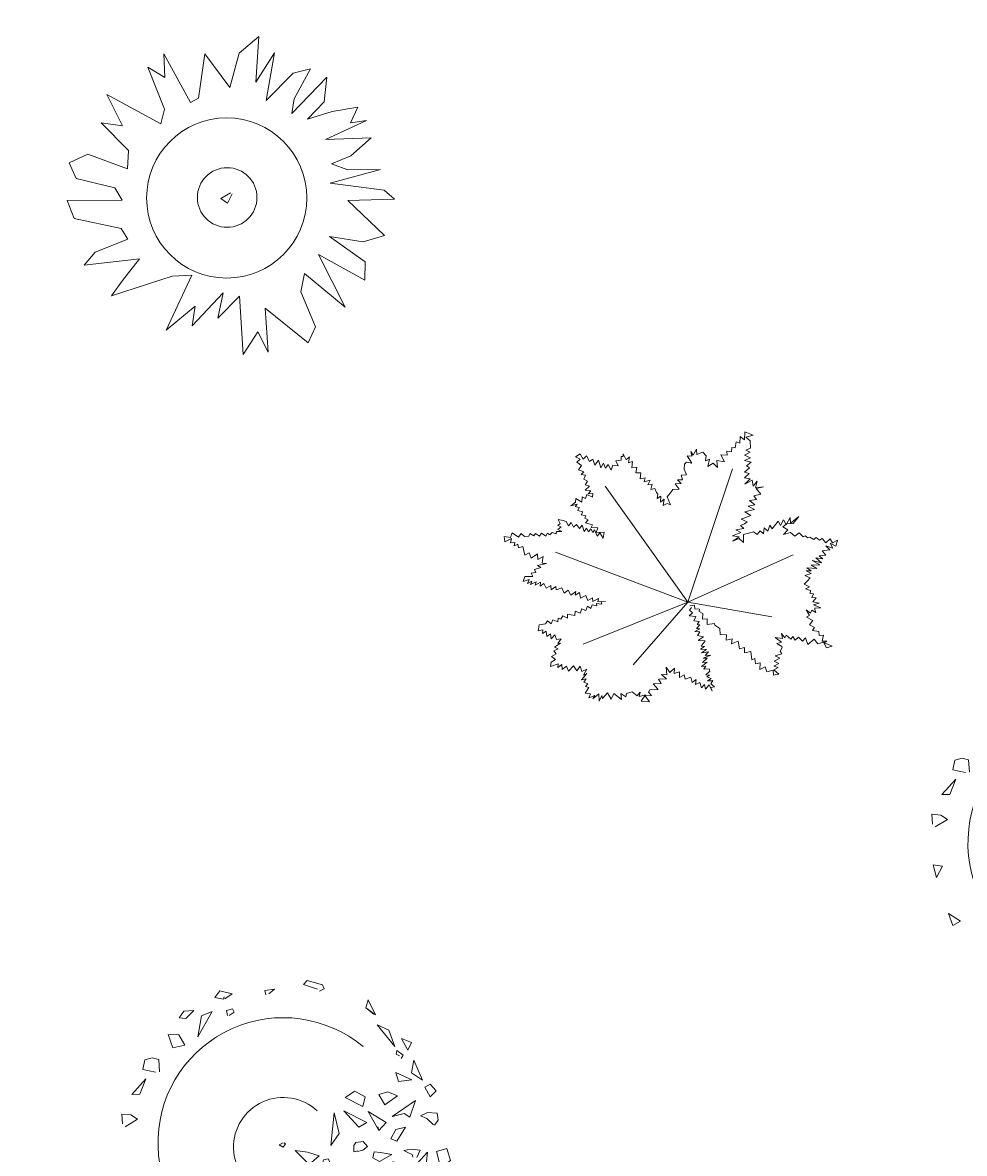
# Model space of a CAD drawing. Units: inches. Extents: x 8049 to 8459, y 820 to 1350.
# Tile 6 of 25: x 8109 to 8132, y 877 to 905. Entities that reach past the tile are written whole.
import ezdxf

# ---------------------------------------------------------------- set-up
doc = ezdxf.new("R2010")
doc.units = ezdxf.units.IN
doc.header["$MEASUREMENT"] = 0
doc.layers.add('A-ANNO-DIMS', color=2, linetype='Continuous', lineweight=18)
doc.layers.add('zelen', color=69, linetype='Continuous', lineweight=13)
doc.styles.get("Standard").update_dxf_attribs({"font": 'arial.ttf'})
doc.dimstyles.get("Standard").update_dxf_attribs({"dimtxt": 0.18, "dimasz": 0.18, "dimexe": 0.18, "dimexo": 0.0625, "dimgap": 0.09, "dimtad": 0, "dimtih": 1, "dimtoh": 1, "dimdec": 4, "dimzin": 0, "dimdsep": 46, "dimtxsty": 'Standard', "dimcen": 0.09, "dimadec": 0, "dimazin": 0, "dimtfac": 1, "dimtdec": 4, "dimtofl": 0, "dimtmove": 0, "dimatfit": 3, "dimfxl": 1, "dimtolj": 1, "dimtzin": 0, "dimarcsym": 0})

# ---------------------------------------------------------------- blocks, each defined once
blk = doc.blocks.new('z_74')
for p, q in [((34.4, 446.7), (93.3, 497)), ((93.3, 497), (83.9, 360.3)), ((-189.4, 445.2), (-110.2, 299.7)), ((-186.5, 374.9), (-189.4, 445.2)), ((-86.8, 312.7), (-67.9, 445.2)), ((-67.9, 445.2), (6.7, 344.6)), ((6.7, 344.6), (34.4, 446.7)), ((83.9, 360.3), (139.6, 447.9)), ((139.6, 447.9), (115.1, 306.1)), ((-237.2, 405.2), (-186.5, 374.9)), ((-188, 280), (-237.2, 405.2)), ((115.1, 306.1), (195.3, 387)), ((191.5, 267.3), (295.2, 375.5)), ((195.3, 387), (247.1, 400.9)), ((247.1, 400.9), (198.5, 310.6)), ((295.2, 375.5), (287.6, 302.1)), ((-359.3, 324.3), (-198.2, 236.1)), ((-312.4, 230.9), (-359.3, 324.3)), ((-110.2, 299.7), (-86.8, 312.7)), ((198.5, 310.6), (191.5, 267.3)), ((-198.2, 236.1), (-188, 280)), ((287.6, 302.1), (238.4, 250.6)), ((238.4, 250.6), (311, 273.7)), ((311, 273.7), (388.2, 286.7)), ((388.2, 286.7), (366, 239.7)), ((-375.9, 239.1), (-312.4, 230.9)), ((-294.6, 157.3), (-375.9, 239.1)), ((413.3, 247), (291.4, 189.7)), ((366, 239.7), (413.3, 247)), ((291.4, 189.7), (427.5, 195.2)), ((427.5, 195.2), (367.5, 141.5)), ((-471.8, 120.9), (-415.6, 146.1)), ((-415.6, 146.1), (-297.6, 102.4)), ((-297.6, 102.4), (-294.6, 157.3)), ((367.5, 141.5), (309.2, 117.3)), ((-450.8, 73.9), (-471.8, 120.9)), ((309.2, 117.3), (358.2, 99.1)), ((-335.1, 45.8), (-450.8, 73.9)), ((455.8, 100.6), (305.4, 59.4)), ((358.2, 99.1), (455.8, 100.6)), ((-313.9, 9.1), (-335.1, 45.8)), ((305.4, 59.4), (466, 38.8)), ((466, 38.8), (497.2, 12.1)), ((-477.4, 8.2), (-313.9, 9.1)), ((-456.4, -45.8), (-477.4, 8.2)), ((8.7, 30.9), (-19.5, 13.9)), ((-19.5, 13.9), (0, 0)), ((0, 0), (13.4, 27.9)), ((497.2, 12.1), (358.2, 8.5)), ((358.2, 8.5), (467.2, -96.1)), ((-316.8, -75.2), (-456.4, -45.8)), ((-296.4, -106.7), (-316.8, -75.2)), ((303.7, -98.8), (410, -174.6)), ((403.6, -114.9), (303.7, -98.8)), ((467.2, -96.1), (403.6, -114.9)), ((-393.7, -146.1), (-296.4, -106.7)), ((-426.7, -184.3), (-393.7, -146.1)), ((-262.6, -165.2), (-426.7, -184.3)), ((-312.7, -229.7), (-262.6, -165.2)), ((271.3, -152.4), (350, -309.1)), ((408.9, -228.8), (271.3, -152.4)), ((410, -174.6), (408.9, -228.8)), ((-165.2, -217.6), (-345.3, -276.1)), ((-345.3, -276.1), (-312.7, -229.7)), ((-182.4, -377.6), (-106.4, -213.9)), ((-106.4, -213.9), (-165.2, -217.6)), ((229.6, -209.7), (218, -264.3)), ((350, -309.1), (229.6, -209.7)), ((-13.1, -266.4), (-105.5, -365.5)), ((-28.9, -341.8), (-13.1, -266.4)), ((218, -264.3), (262, -367.6)), ((35.8, -276.7), (-28.9, -341.8)), ((46.6, -450.6), (35.8, -276.7)), ((-96.5, -306.1), (-182.4, -377.6)), ((-105.5, -365.5), (-96.5, -306.1)), ((111.6, -312.4), (120.9, -443.4)), ((240.1, -415.5), (111.6, -312.4)), ((262, -367.6), (240.1, -415.5)), ((90.1, -383.4), (46.6, -450.6)), ((120.9, -443.4), (90.1, -383.4))]:
    blk.add_line(p, q)
for centre, radius in [((-2.5, 15.8), 238.5), ((-1.1, 17.1), 88.8)]:
    blk.add_circle(centre, radius)
blk = doc.blocks.new('z_85')
for p, q in [((168.5, 483.9), (169.7, 507.5)), ((169.7, 507.5), (194.7, 497.5)), ((140.4, 459.9), (144.1, 478.3)), ((144.1, 478.3), (154.8, 474.2)), ((154.8, 474.2), (155.6, 493.8)), ((155.6, 493.8), (168.5, 483.9)), ((194.7, 497.5), (173, 491.4)), ((173, 491.4), (185.2, 481.2)), ((185.2, 481.2), (186.9, 458.5)), ((-334.5, 433), (-320.5, 441.8)), ((-320.5, 441.8), (-312.2, 426.3)), ((-192.6, 433.8), (-192.5, 442.2)), ((-192.5, 442.2), (-183.3, 424.5)), ((8.4, 449), (15.4, 438)), ((11.7, 434.9), (8.4, 449)), ((15.4, 438), (25.6, 455.6)), ((25.6, 455.6), (26.4, 439.7)), ((26.4, 439.7), (44.1, 447.4)), ((44.1, 447.4), (54.4, 436.3)), ((98.5, 438.8), (116.6, 438)), ((108.9, 418.4), (98.5, 438.8)), ((116.1, 450.2), (130, 447.6)), ((116.6, 438), (116.1, 450.2)), ((130, 447.6), (130.9, 460.7)), ((130.9, 460.7), (140.4, 459.9)), ((185.1, 447.3), (169, 438)), ((169, 438), (186.4, 430.3)), ((186.9, 458.5), (172.1, 453.2)), ((172.1, 453.2), (185.1, 447.3)), ((-320.3, 426.3), (-334.5, 433)), ((-331, 417), (-320.3, 426.3)), ((-316.9, 407.2), (-331, 417)), ((-325.3, 394.5), (-316.9, 407.2)), ((-312.2, 426.3), (-302, 436.4)), ((-302, 436.4), (-292.5, 418.9)), ((-292.5, 418.9), (-282.7, 426.1)), ((-282.7, 426.1), (-277, 408.1)), ((-277, 408.1), (-266.3, 423.5)), ((-266.3, 423.5), (-258.7, 400.7)), ((-258.7, 400.7), (-250.8, 414.2)), ((-250.8, 414.2), (-244.9, 399.8)), ((-244.9, 399.8), (-237.2, 410.8)), ((-237.2, 410.8), (-228.5, 393.9)), ((-228.5, 393.9), (-223.5, 408.6)), ((-223.5, 408.6), (-207.8, 406.4)), ((-214.2, 421.3), (-198.5, 423)), ((-207.8, 406.4), (-214.2, 421.3)), ((-198.5, 423), (-198.2, 434.1)), ((-198.2, 434.1), (-192.6, 433.8)), ((-183.3, 424.5), (-173.3, 433.2)), ((-173.3, 433.2), (-176.4, 415.5)), ((-176.4, 415.5), (-165.1, 418.9)), ((-165.1, 418.9), (-166.4, 400.3)), ((-10.8, 396), (-9.6, 410.9)), ((-9.6, 410.9), (-3.8, 416.9)), ((-3.8, 416.9), (11.4, 414.5)), ((-2.1, 435.8), (11.7, 434.9)), ((11.4, 414.5), (-2.1, 435.8)), ((54.4, 436.3), (52.3, 421.7)), ((52.3, 421.7), (64.6, 426)), ((64.6, 426), (59.8, 403.9)), ((59.8, 403.9), (75.6, 414.2)), ((75.6, 414.2), (88.3, 401.4)), ((86.4, 422.5), (108.9, 418.4)), ((88.3, 401.4), (86.4, 422.5)), ((186.4, 430.3), (169.1, 422.7)), ((169.1, 422.7), (188.1, 417.5)), ((188.1, 417.5), (174.5, 406.5)), ((174.5, 406.5), (183.6, 400.7)), ((-309.5, 388.7), (-325.3, 394.5)), ((-317.2, 380.4), (-309.5, 388.7)), ((-305.1, 378.2), (-317.2, 380.4)), ((-309.5, 366.8), (-305.1, 378.2)), ((-166.4, 400.3), (-152.4, 402.8)), ((-152.4, 402.8), (-154.8, 385.2)), ((-154.8, 385.2), (-139.8, 385.6)), ((-139.8, 385.6), (-142, 367.5)), ((-142, 367.5), (-126.8, 370.7)), ((-126.8, 370.7), (-129.7, 358.9)), ((-19.9, 378.2), (-4.1, 379.1)), ((-16.4, 364.7), (-19.9, 378.2)), ((-4.1, 379.1), (-10.8, 396)), ((0, 0), (132.7, 397)), ((182.7, 383.5), (168.5, 371)), ((168.5, 371), (185.5, 367.5)), ((183.6, 400.7), (169.1, 387.1)), ((169.1, 387.1), (182.7, 383.5)), ((-299.2, 360.3), (-309.5, 366.8)), ((-305.9, 349.8), (-299.2, 360.3)), ((-292.6, 345.9), (-305.9, 349.8)), ((-305.3, 333.9), (-292.6, 345.9)), ((0, 0), (-245.8, 345.3)), ((-129.7, 358.9), (-112.6, 364.1)), ((-112.6, 364.1), (-118.7, 349.7)), ((-118.7, 349.7), (-106.5, 351.7)), ((-106.5, 351.7), (-110.4, 335.8)), ((-110.4, 335.8), (-98.6, 339.2)), ((-98.6, 339.2), (-92.9, 326.8)), ((-45, 336.2), (-26.1, 337)), ((-37.5, 352.7), (-19.6, 354.2)), ((-26.1, 337), (-37.5, 352.7)), ((-31.2, 364.3), (-16.4, 364.7)), ((-19.6, 354.2), (-31.2, 364.3)), ((185.5, 367.5), (169.7, 351.3)), ((169.7, 351.3), (191.1, 364.1)), ((191.1, 364.1), (194, 345.3)), ((194, 345.3), (206.3, 360.8)), ((206.3, 360.8), (201.7, 341.2)), ((201.7, 341.2), (224.8, 344.2)), ((224.8, 344.2), (203.2, 339.2)), ((203.2, 339.2), (217.5, 321.8)), ((-334.3, 298.5), (-333.4, 308.7)), ((-333.4, 308.7), (-315.2, 298.3)), ((-315.2, 298.3), (-314.9, 314.1)), ((-314.9, 314.1), (-305, 309.4)), ((-288.9, 332.3), (-305.3, 333.9)), ((-305, 309.4), (-300.9, 321)), ((-300.9, 321), (-284.3, 312.7)), ((-296.8, 323.1), (-288.9, 332.3)), ((-283.1, 324), (-296.8, 323.1)), ((-284.3, 312.7), (-283.1, 324)), ((-92.9, 326.8), (-89.6, 322.3)), ((-89.6, 322.3), (-91.1, 309)), ((-91.1, 309), (-80.4, 316.3)), ((-80.4, 316.3), (-81.2, 298.5)), ((-81.2, 298.5), (-70.2, 306.6)), ((-70.2, 306.6), (-73.6, 287.8)), ((-61.6, 314), (-48.8, 329.6)), ((-51.7, 290.2), (-61.6, 314)), ((-48.8, 329.6), (-45, 336.2)), ((204.7, 306.3), (183.1, 303.2)), ((183.1, 303.2), (199.8, 290.5)), ((217.5, 321.8), (196.8, 317.3)), ((196.8, 317.3), (204.7, 306.3)), ((-348.8, 287.5), (-334.3, 298.5)), ((-329.7, 291.9), (-348.8, 287.5)), ((-335.7, 285.2), (-329.7, 291.9)), ((-323.9, 282.5), (-335.7, 285.2)), ((-327.7, 273.4), (-323.9, 282.5)), ((-312.5, 269.8), (-327.7, 273.4)), ((-318.1, 260.9), (-312.5, 269.8)), ((-73.6, 287.8), (-62, 294.6)), ((-62, 294.6), (-51.7, 290.2)), ((198, 276.2), (169.3, 269.4)), ((199.8, 290.5), (179.5, 286.4)), ((179.5, 286.4), (198, 276.2)), ((-386.6, 246.8), (-370.9, 243.8)), ((-380.3, 234.1), (-386.6, 246.8)), ((-370.9, 243.8), (-362.5, 240.1)), ((-362.5, 240.1), (-355.4, 227.7)), ((-355.4, 227.7), (-347.7, 237.1)), ((-347.7, 237.1), (-340.1, 223.9)), ((-303.5, 257.1), (-318.1, 260.9)), ((-306.9, 250.2), (-303.5, 257.1)), ((-296.5, 245.4), (-306.9, 250.2)), ((-304.8, 236.9), (-296.5, 245.4)), ((-284, 230.8), (-304.8, 236.9)), ((187.9, 258.2), (158.6, 247.3)), ((158.6, 247.3), (176.5, 239.3)), ((176.5, 239.3), (169.1, 234)), ((169.3, 269.4), (187.9, 258.2)), ((251.2, 218.3), (269.1, 241.8)), ((269.1, 241.8), (276.1, 228.2)), ((276.1, 228.2), (284.6, 245.4)), ((284.6, 245.4), (292.5, 230.8)), ((292.5, 230.8), (304.2, 252.6)), ((304.2, 252.6), (305.4, 235.8)), ((305.4, 235.8), (330.6, 255.3)), ((330.6, 255.3), (314, 234.4)), ((-527.9, 192.6), (-523, 206.4)), ((-523, 206.4), (-504.7, 194.2)), ((-504.7, 194.2), (-496.5, 204.8)), ((-496.5, 204.8), (-486, 196.2)), ((-473.8, 197.3), (-470.6, 205)), ((-470.6, 205), (-459, 197.9)), ((-459, 197.9), (-453.2, 204.7)), ((-453.2, 204.7), (-441.7, 197.3)), ((-441.7, 197.3), (-436, 206.1)), ((-436, 206.1), (-423, 196.7)), ((-423, 196.7), (-417.9, 205.5)), ((-417.9, 205.5), (-411.3, 200.8)), ((-411.3, 200.8), (-403.9, 207.3)), ((-403.9, 207.3), (-392, 203.9)), ((-392, 203.9), (-391, 210.5)), ((-391, 210.5), (-375.1, 210.9)), ((-387.5, 216.4), (-377.3, 224.9)), ((-375.1, 210.9), (-387.5, 216.4)), ((-387.2, 228.2), (-380.3, 234.1)), ((-377.3, 224.9), (-387.2, 228.2)), ((-340.1, 223.9), (-331.2, 232.1)), ((-331.2, 232.1), (-323, 219.9)), ((-323, 219.9), (-314.9, 229.4)), ((-314.9, 229.4), (-308.7, 210.5)), ((-308.7, 210.5), (-301.4, 220.5)), ((-301.4, 220.5), (-296.2, 209.5)), ((-296.2, 209.5), (-288.7, 218.5)), ((-288.7, 218.5), (-282.8, 208)), ((-287.5, 222.7), (-284, 230.8)), ((-267.9, 221.3), (-287.5, 222.7)), ((-282.8, 208), (-278.3, 215.3)), ((-278.3, 215.3), (-269.6, 197)), ((-272.7, 208.1), (-267.9, 221.3)), ((-249.1, 208.6), (-272.7, 208.1)), ((-269.6, 197), (-261.6, 206.7)), ((-261.6, 206.7), (-252.6, 191.1)), ((-252.6, 191.1), (-249.1, 208.6)), ((157.5, 207.7), (133, 198.3)), ((166.6, 220), (142.5, 215.8)), ((142.5, 215.8), (157.5, 207.7)), ((169.1, 234), (156.5, 228.6)), ((156.5, 228.6), (166.6, 220)), ((165.5, 178.4), (166.1, 202.2)), ((166.1, 202.2), (195.8, 210)), ((195.8, 210), (206.3, 202.3)), ((206.3, 202.3), (214.9, 212.7)), ((214.9, 212.7), (225, 203.7)), ((225, 203.7), (227.4, 221.4)), ((227.4, 221.4), (237.6, 211.9)), ((237.6, 211.9), (244, 229.6)), ((244, 229.6), (251.2, 218.3)), ((291.9, 231.3), (282.8, 224.3)), ((282.8, 224.3), (297.7, 215.3)), ((297.7, 215.3), (285.2, 201.4)), ((285.2, 201.4), (305.7, 207.8)), ((294, 233.8), (291.9, 231.3)), ((314, 234.4), (294, 233.8)), ((305.7, 207.8), (318.4, 196.7)), ((318.4, 196.7), (331.5, 207.2)), ((331.5, 207.2), (343.4, 195.3)), ((-547.4, 195.4), (-527.9, 192.6)), ((-544.7, 179.5), (-547.4, 195.4)), ((-524.7, 189.5), (-544.7, 179.5)), ((-528.5, 176.6), (-524.7, 189.5)), ((-515.5, 177.6), (-528.5, 176.6)), ((-516.7, 167.9), (-515.5, 177.6)), ((-506.3, 173.2), (-516.7, 167.9)), ((-504.7, 162.4), (-506.3, 173.2)), ((-486, 196.2), (-473.8, 197.3)), ((133, 198.3), (152.7, 194.8)), ((152.7, 194.8), (134.2, 181.8)), ((134.2, 181.8), (152.3, 190.3)), ((152.3, 190.3), (165.5, 178.4)), ((343.4, 195.3), (349.2, 197.8)), ((349.2, 197.8), (357.1, 191.7)), ((357.1, 191.7), (363.4, 194)), ((363.4, 194), (375.4, 187.3)), ((375.4, 187.3), (381.6, 192.9)), ((381.6, 192.9), (391.6, 185.1)), ((391.6, 185.1), (399.5, 189.8)), ((399.5, 189.8), (410.7, 177.1)), ((410.7, 177.1), (423.8, 189)), ((423.8, 189), (430.9, 177.3)), ((423.8, 175.6), (431.6, 161.5)), ((440.2, 166.6), (423.8, 175.6)), ((430.9, 177.3), (445.2, 185.4)), ((445.2, 185.4), (440.2, 166.6)), ((-491.4, 165.7), (-504.7, 162.4)), ((-484.9, 140.6), (-491.4, 165.7)), ((-472, 147), (-484.9, 140.6)), ((-466.4, 131.1), (-472, 147)), ((-447.4, 143.9), (-466.4, 131.1)), ((-446.4, 127.5), (-447.4, 143.9)), ((-431.2, 136.1), (-446.4, 127.5)), ((-432.5, 124.7), (-431.2, 136.1)), ((0, 0), (-394.4, 149.4)), ((0, 0), (313.9, 140.8)), ((410.7, 140.5), (391.1, 138)), ((391.1, 138), (402.3, 129)), ((422.9, 156), (399.8, 152.7)), ((399.8, 152.7), (410.7, 140.5)), ((410.7, 167.7), (422.9, 156)), ((431.6, 161.5), (410.7, 167.7)), ((-456.8, 97.3), (-437.9, 103.7)), ((-447.3, 109), (-420.9, 115.7)), ((-437.9, 103.7), (-447.3, 109)), ((-433.6, 116.8), (-432.5, 124.7)), ((-420.9, 115.7), (-433.6, 116.8)), ((354.4, 102.3), (367.3, 93.6)), ((384, 100.5), (354.4, 102.3)), ((392.9, 111.3), (367, 110.4)), ((367, 110.4), (384, 100.5)), ((370, 124.5), (392.9, 111.3)), ((397.4, 117.9), (370, 124.5)), ((380.7, 131.9), (397.4, 117.9)), ((402.3, 129), (380.7, 131.9)), ((-490.1, 61.5), (-485.7, 76.6)), ((-472.7, 67.7), (-490.1, 61.5)), ((-485.7, 76.6), (-461.1, 77.2)), ((-477.3, 56.2), (-472.7, 67.7)), ((-466.3, 86.6), (-452.6, 88.2)), ((-461.1, 77.2), (-466.3, 86.6)), ((-452.6, 88.2), (-456.8, 97.3)), ((367.5, 85.5), (348.2, 79.7)), ((348.2, 79.7), (364, 72.5)), ((367.3, 93.6), (352.7, 93.5)), ((352.7, 93.5), (367.5, 85.5)), ((364, 72.5), (355.3, 62.8)), ((-464.1, 63.3), (-477.3, 56.2)), ((-468.4, 52.6), (-464.1, 63.3)), ((-452, 61.1), (-468.4, 52.6)), ((-455.1, 51.2), (-452, 61.1)), ((-439, 59.8), (-455.1, 51.2)), ((-439.5, 47.5), (-439, 59.8)), ((-428.5, 56.1), (-439.5, 47.5)), ((-421.5, 42.4), (-428.5, 56.1)), ((-408.4, 49.5), (-421.5, 42.4)), ((-406.6, 37.3), (-408.4, 49.5)), ((-393.5, 46.8), (-406.6, 37.3)), ((-392.2, 37), (-393.5, 46.8)), ((-375.3, 43.4), (-392.2, 37)), ((-368.7, 27.4), (-375.3, 43.4)), ((-356.3, 36.3), (-368.7, 27.4)), ((-348.5, 20.8), (-356.3, 36.3)), ((355.3, 62.8), (346.4, 53.6)), ((346.4, 53.6), (362.3, 46.4)), ((362.3, 46.4), (350.4, 40.1)), ((350.4, 40.1), (365.4, 35.2)), ((365.4, 35.2), (364.6, 26)), ((-333.9, 32.3), (-348.5, 20.8)), ((-335.5, 21.5), (-333.9, 32.3)), ((-322.4, 29.1), (-335.5, 21.5)), ((-319.9, 12.2), (-322.4, 29.1)), ((-303.8, 20), (-319.9, 12.2)), ((0, 0), (-312.2, -125)), ((-297.7, 5.3), (-303.8, 20)), ((-284.2, 12.8), (-297.7, 5.3)), ((-282.8, 2.5), (-284.2, 12.8)), ((-266.1, 11.6), (-282.8, 2.5)), ((-268.5, 0.9), (-266.1, 11.6)), ((-245.2, 1.9), (-268.5, 0.9)), ((-258.6, 1.3), (-245.2, 1.9)), ((-256.6, -5.5), (-258.6, 1.3)), ((0, 0), (-163.1, -186)), ((0, 0), (249.7, -43.2)), ((364.6, 26), (373.9, 25.2)), ((373.9, 25.2), (368.8, 14.6)), ((368.8, 14.6), (381.5, 13.5)), ((381.5, 13.5), (372.3, 1.1)), ((372.3, 1.1), (390.8, -3.1)), ((-337, -39.8), (-335.4, -26.5)), ((-335.4, -26.5), (-320, -32.7)), ((-320, -32.7), (-316.6, -19.6)), ((-316.6, -19.6), (-303.5, -24.4)), ((-303.5, -24.4), (-299.1, -12.1)), ((-299.1, -12.1), (-288.4, -18.9)), ((-288.4, -18.9), (-284.9, -7.8)), ((-284.9, -7.8), (-270.6, -10.5)), ((-272, -3.8), (-256.6, -5.5)), ((-270.6, -10.5), (-272, -3.8)), ((14.2, -31.5), (3.8, -40.4)), ((11, -15.5), (4.4, -23.3)), ((4.4, -23.3), (14.2, -31.5)), ((19.4, -9.1), (6, -11.1)), ((20.6, -19.7), (19.4, -9.1)), ((34.5, -21), (20.6, -19.7)), ((33.9, -27.7), (34.5, -21)), ((44.7, -33.5), (33.9, -27.7)), ((43.2, -50.4), (44.7, -33.5)), ((352.1, -22.6), (362.5, -39.2)), ((365.2, -32.7), (352.1, -22.6)), ((368.7, -23.2), (365.2, -32.7)), ((380.7, -30.1), (368.7, -23.2)), ((390.8, -3.1), (374.2, -7.2)), ((374.2, -7.2), (396.2, -16.9)), ((378.3, -17.7), (377.9, -21.9)), ((377.9, -21.9), (380.7, -30.1)), ((396.2, -16.9), (378.3, -17.7)), ((-445.6, -85.2), (-442.8, -66.9)), ((-442.8, -66.9), (-423.6, -64.7)), ((-423.6, -64.7), (-418.1, -55.3)), ((-418.1, -55.3), (-406.6, -63.9)), ((-406.6, -63.9), (-402.1, -52.8)), ((-402.1, -52.8), (-387.5, -58.3)), ((-387.5, -58.3), (-386, -47.3)), ((-386, -47.3), (-378.3, -50.6)), ((-378.3, -50.6), (-371.8, -40.4)), ((-371.8, -40.4), (-358.3, -47.6)), ((-358.6, -35.2), (-337, -39.8)), ((-358.3, -47.6), (-358.6, -35.2)), ((3.8, -40.4), (23.3, -42)), ((23.3, -42), (17.8, -55.3)), ((17.8, -55.3), (33.3, -57.2)), ((35.8, -67.3), (26.2, -78.5)), ((33.3, -57.2), (27.6, -66.1)), ((27.6, -66.1), (35.8, -67.3)), ((57.8, -49.8), (43.2, -50.4)), ((57.8, -66.7), (57.8, -49.8)), ((79.4, -63.3), (57.8, -66.7)), ((80.6, -68.6), (79.4, -63.3)), ((362.5, -39.2), (352.9, -44.5)), ((352.9, -44.5), (372.4, -54.8)), ((372.4, -54.8), (362.2, -67.3)), ((362.2, -67.3), (377.4, -74.9)), ((-431.8, -81.7), (-445.6, -85.2)), ((-433, -93.3), (-431.8, -81.7)), ((-421.5, -86.1), (-433, -93.3)), ((-420.3, -102.3), (-421.5, -86.1)), ((-408.9, -93.6), (-420.3, -102.3)), ((-406.5, -108.7), (-408.9, -93.6)), ((-396.2, -96.8), (-406.5, -108.7)), ((-391.4, -111), (-396.2, -96.8)), ((35.4, -79.2), (20.9, -86.9)), ((20.9, -86.9), (36.1, -88.5)), ((26.2, -78.5), (35.4, -79.2)), ((36.1, -88.5), (28.2, -99.3)), ((28.2, -99.3), (46.8, -102.9)), ((95, -77.7), (80.6, -68.6)), ((96.5, -95.7), (95, -77.7)), ((114.9, -96.9), (96.5, -95.7)), ((113.9, -113.2), (114.9, -96.9)), ((279.1, -92.7), (281.6, -108.4)), ((288.4, -105.6), (279.1, -92.7)), ((292.3, -97.7), (288.4, -105.6)), ((306.3, -109.8), (292.3, -97.7)), ((377.4, -74.9), (371.4, -84.3)), ((371.4, -84.3), (390.2, -87.1)), ((390.2, -87.1), (391, -98.7)), ((391, -98.7), (403.6, -97.7)), ((403.6, -97.7), (399.4, -115.7)), ((-396.7, -133.3), (-378.8, -121.8)), ((-386, -138.6), (-396.7, -133.3)), ((-377.3, -108.5), (-391.4, -111)), ((-387.6, -122.5), (-377.3, -108.5)), ((-378.8, -121.8), (-387.6, -122.5)), ((31.9, -112.9), (31.3, -114)), ((31.3, -114), (51.4, -114.8)), ((46.8, -102.9), (31.9, -112.9)), ((49.4, -132), (38, -139.7)), ((51.4, -114.8), (39.8, -130.3)), ((39.8, -130.3), (49.4, -132)), ((131.6, -109.3), (113.9, -113.2)), ((129.5, -124.2), (131.6, -109.3)), ((150, -116), (129.5, -124.2)), ((153.5, -138.6), (150, -116)), ((168.2, -134.7), (153.5, -138.6)), ((168.7, -151.1), (168.2, -134.7)), ((259.9, -104.5), (278.9, -118.5)), ((281.6, -108.4), (259.9, -104.5)), ((278.9, -118.5), (264.8, -122.8)), ((264.8, -122.8), (279.4, -131.9)), ((280.4, -134.4), (275.3, -145.6)), ((279.4, -131.9), (280.4, -134.4)), ((312.3, -101.9), (306.3, -109.8)), ((319.1, -112.6), (312.3, -101.9)), ((329.4, -104.1), (319.1, -112.6)), ((341.7, -115.9), (329.4, -104.1)), ((350.6, -106.3), (341.7, -115.9)), ((357.5, -125.6), (350.6, -106.3)), ((375.9, -109.5), (357.5, -125.6)), ((386.6, -123.9), (375.9, -109.5)), ((403.8, -118.5), (386.6, -123.9)), ((399.4, -115.7), (414.2, -115.6)), ((413.1, -135.8), (403.8, -118.5)), ((414.2, -115.6), (406.2, -120.7)), ((406.2, -120.7), (430, -130.9)), ((430, -130.9), (413.1, -135.8)), ((-405.7, -161.9), (-391.7, -153.5)), ((-394, -170.7), (-405.7, -161.9)), ((-399.4, -144.9), (-386, -138.6)), ((-391.7, -153.5), (-399.4, -144.9)), ((38, -139.7), (55.7, -140.9)), ((55.7, -140.9), (40.8, -150.5)), ((40.8, -150.5), (61.7, -147.7)), ((57.7, -166.9), (43.5, -179.6)), ((67.9, -157.4), (45.5, -166.6)), ((45.5, -166.6), (57.7, -166.9)), ((61.7, -147.7), (51.2, -158.2)), ((51.2, -158.2), (67.9, -157.4)), ((187.2, -147), (168.7, -151.1)), ((190.4, -171.9), (187.2, -147)), ((199.5, -167.6), (190.4, -171.9)), ((201.2, -183.5), (199.5, -167.6)), ((273.9, -166.2), (257.2, -175.1)), ((279.5, -153.9), (259.5, -159.1)), ((259.5, -159.1), (273.9, -166.2)), ((275.3, -145.6), (279.5, -153.9)), ((-408.7, -191.2), (-407.1, -178.7)), ((-386.3, -183.7), (-408.7, -191.2)), ((-407.1, -178.7), (-394, -170.7)), ((-386.9, -194.2), (-386.3, -183.7)), ((-375, -185.4), (-386.9, -194.2)), ((-374.4, -200.4), (-375, -185.4)), ((-361, -190), (-374.4, -200.4)), ((-355.6, -205.5), (-361, -190)), ((-340.1, -188.9), (-355.6, -205.5)), ((-331, -204.2), (-340.1, -188.9)), ((-320.5, -190.1), (-331, -204.2)), ((-315.8, -206.4), (-320.5, -190.1)), ((-300.9, -199.4), (-315.8, -206.4)), ((-311, -217.5), (-300.9, -199.4)), ((-64.5, -193.4), (-63.1, -216.4)), ((-54.1, -209.7), (-64.5, -193.4)), ((-39.9, -196.5), (-54.1, -209.7)), ((-40.4, -212.5), (-39.9, -196.5)), ((57.1, -178.7), (40.5, -191.1)), ((40.5, -191.1), (53.9, -190.4)), ((43.5, -179.6), (57.1, -178.7)), ((53.9, -190.4), (47.9, -199)), ((47.9, -199), (63.4, -198.7)), ((63.4, -198.7), (65.1, -205.6)), ((215.4, -180.2), (201.2, -183.5)), ((214.3, -200.6), (215.4, -180.2)), ((229.7, -192.5), (214.3, -200.6)), ((235.5, -207.5), (229.7, -192.5)), ((253.5, -202), (235.5, -207.5)), ((255.4, -217.1), (253.5, -202)), ((270.6, -182.1), (255.6, -190.7)), ((255.6, -190.7), (268.7, -194.5)), ((268.7, -194.5), (256, -201.4)), ((256, -201.4), (270.6, -214.1)), ((257.2, -175.1), (270.6, -182.1)), ((-316.4, -230.7), (-301.2, -212.5)), ((-303, -227.7), (-316.4, -230.7)), ((-301.2, -212.5), (-311, -217.5)), ((-309.9, -238.3), (-303, -227.7)), ((-63.4, -228.2), (-87.9, -229.1)), ((-87.9, -229.1), (-79.8, -242)), ((-78.5, -215.2), (-63.4, -228.2)), ((-63.1, -216.4), (-78.5, -215.2)), ((-25.3, -207.7), (-40.4, -212.5)), ((-25.3, -223.8), (-25.3, -207.7)), ((-10.7, -215.8), (-25.3, -223.8)), ((-8.3, -228.6), (-10.7, -215.8)), ((8.9, -223.5), (-8.3, -228.6)), ((12.7, -238.7), (8.9, -223.5)), ((24.7, -230.5), (12.7, -238.7)), ((23, -244.8), (24.7, -230.5)), ((65.1, -205.6), (53.6, -216.1)), ((53.6, -216.1), (64.9, -216.9)), ((64.9, -216.9), (56, -222.4)), ((56, -222.4), (69.4, -226.9)), ((69.4, -226.9), (58.1, -234.3)), ((58.1, -234.3), (70.9, -234.4)), ((73.9, -233.5), (67.9, -243.4)), ((70.9, -234.4), (73.9, -233.5)), ((270.6, -214.1), (255.4, -217.1)), ((-298.3, -242.6), (-309.9, -238.3)), ((-305.3, -270.9), (-295, -254.3)), ((-304.7, -251.3), (-298.3, -242.6)), ((-295, -254.3), (-304.7, -251.3)), ((-166.3, -266.5), (-182.4, -271.4)), ((-151.2, -278.6), (-166.3, -266.5)), ((-142.3, -267.5), (-151.2, -278.6)), ((-144.6, -280.3), (-142.3, -267.5)), ((-113.1, -261.1), (-117.3, -267.5)), ((-117.3, -267.5), (-107.8, -278)), ((-88.9, -260), (-113.1, -261.1)), ((-79.8, -242), (-103.3, -242.6)), ((-103.3, -242.6), (-88.9, -260)), ((35.5, -238.8), (23, -244.8)), ((40.7, -254.5), (35.5, -238.8)), ((49.8, -244.9), (40.7, -254.5)), ((52.7, -259.2), (49.8, -244.9)), ((63.6, -245.9), (52.7, -259.2)), ((72.4, -265), (63.6, -245.9)), ((67.9, -243.4), (79.4, -252.4)), ((79.4, -252.4), (68.2, -253.9)), ((68.2, -253.9), (72.4, -265)), ((-290.1, -273.1), (-305.3, -270.9)), ((-294.6, -284.2), (-290.1, -273.1)), ((-277.1, -277.7), (-294.6, -284.2)), ((-264.9, -273), (-283.1, -288.1)), ((-283.1, -288.1), (-277.1, -277.7)), ((-264.3, -294.3), (-264.9, -273)), ((-256.6, -277.5), (-264.3, -294.3)), ((-254.5, -286.6), (-256.6, -277.5)), ((-239.6, -270.1), (-254.5, -286.6)), ((-228.6, -289.1), (-239.6, -270.1)), ((-220, -272), (-228.6, -289.1)), ((-197.9, -289.9), (-220, -272)), ((-199.2, -272), (-197.9, -289.9)), ((-184.2, -282), (-199.2, -272)), ((-182.4, -271.4), (-184.2, -282)), ((-126.2, -276.2), (-144.6, -280.3)), ((-138.9, -294.9), (-126.2, -276.2)), ((-114.3, -296.8), (-138.9, -294.9)), ((-107.8, -278), (-127.3, -279.2)), ((-127.3, -279.2), (-114.3, -296.8))]:
    blk.add_line(p, q)
blk = doc.blocks.new('z_66')
for p, q in [((83.2, 488.9), (72.7, 477.7)), ((72.7, 477.7), (96.4, 469.7)), ((129.8, 476.2), (83.2, 488.9)), ((134, 464.6), (129.8, 476.2)), ((-176.4, 458.5), (-191.7, 438.6)), ((-191.7, 438.6), (-165.6, 433.5)), ((-139.2, 449.4), (-176.4, 458.5)), ((-165.6, 433.5), (-163.6, 441.1)), ((-161.1, 434.6), (-139.2, 449.4)), ((-13.6, 463.6), (-42.5, 459.2)), ((-42.5, 459.2), (-39.3, 446.9)), ((-30.3, 449.4), (-13.6, 463.6)), ((96.4, 469.7), (114.5, 463.9)), ((114.5, 463.9), (114.5, 463.9)), ((120.4, 457.8), (134, 464.6)), ((-165.6, 433.5), (-165.6, 433.5)), ((-138.9, 404.9), (-156.9, 400.2)), ((-133.3, 394.8), (-138.9, 404.9)), ((265.2, 432.1), (258.2, 407.5)), ((258.2, 407.5), (287.4, 387.2)), ((258.2, 407.5), (281.9, 388.6)), ((287.4, 387.2), (265.2, 432.1)), ((-283.6, 397.7), (-297.2, 378.2)), ((-297.2, 378.2), (-277.7, 376)), ((-254, 399.9), (-283.6, 397.7)), ((-277.7, 376), (-272.8, 380.7)), ((-272.8, 380.7), (-254, 399.9)), ((-241.9, 321.7), (-199.1, 397.3)), ((-231.4, 383.6), (-241.9, 321.7)), ((-199.1, 397.3), (-231.4, 383.6)), ((-156.9, 400.2), (-153.8, 385.4)), ((-148.6, 384.7), (-133.3, 394.8)), ((281.9, 388.6), (281.9, 388.6)), ((344.2, 293.1), (292, 357.2)), ((292, 357.2), (326.8, 341.2)), ((326.8, 341.2), (344.2, 293.1)), ((-330.3, 328.9), (-298.6, 327.1)), ((-316, 288.8), (-330.3, 328.9)), ((-298.6, 327.1), (-280.8, 297.1)), ((383.1, 281.9), (364.4, 316.3)), ((364.4, 316.3), (394.6, 305.1)), ((394.6, 305.1), (383.1, 281.9)), ((-280.8, 297.1), (-316, 288.8)), ((350.8, 280.8), (348.7, 270.3)), ((348.7, 270.3), (358.8, 264.5)), ((369.2, 266.7), (350.8, 280.8)), ((-399.2, 252.6), (-405.8, 224)), ((-377.9, 259.1), (-399.2, 252.6)), ((-358.4, 254), (-377.9, 259.1)), ((-356, 217.5), (-358.4, 254)), ((358.8, 264.5), (358.8, 264.5)), ((363.3, 256.6), (369.2, 266.7)), ((400.9, 251.9), (393.9, 214.6)), ((426.6, 192.2), (400.9, 251.9)), ((-405.8, 224), (-368.2, 216.4)), ((-368.2, 216.4), (-368.2, 216.4)), ((348, 215.7), (356, 188.9)), ((395.3, 193.2), (348, 215.7)), ((393.9, 214.6), (426.6, 192.2)), ((-396.4, 196.1), (-438.1, 150.2)), ((-414.8, 150.9), (-396.4, 196.1)), ((356, 188.9), (395.3, 193.2)), ((450, 180.6), (434.3, 171.2)), ((434.3, 171.2), (449.6, 142.6)), ((467.7, 160.3), (450, 180.6)), ((-438.1, 150.2), (-414.8, 150.9)), ((225.2, 159.9), (197, 140.8)), ((197, 140.8), (249.5, 113.6)), ((256.8, 142.6), (225.2, 159.9)), ((249.5, 113.6), (256.8, 142.6)), ((323.6, 157.8), (297.5, 149.8)), ((297.5, 149.8), (314.6, 119.4)), ((314.6, 119.4), (352.9, 145.5)), ((352.9, 145.5), (323.6, 157.8)), ((449.6, 142.6), (467.7, 160.3)), ((193.1, 101.3), (238, 52.1)), ((261.7, 66.6), (193.1, 101.3)), ((336.9, 84.3), (405.8, 131.7)), ((405.8, 131.7), (389.8, 82.1)), ((-468.4, 91.6), (-466.3, 62.6)), ((-441.6, 89), (-468.4, 91.6)), ((-458.3, 53.9), (-421.1, 76)), ((-421.1, 76), (-441.6, 89)), ((164.3, 94.8), (154.2, -2.2)), ((178.9, 33.3), (164.3, 94.8)), ((265.2, 98.8), (297.2, 42.7)), ((318.8, 66.2), (265.2, 98.8)), ((372.7, 93), (336.9, 84.3)), ((389.8, 82.1), (372.7, 93)), ((441.6, 95.9), (420.7, 86.5)), ((420.7, 86.5), (440.2, 78.5)), ((440.2, 78.5), (459.7, 59.7)), ((470.5, 93.7), (441.6, 95.9)), ((463.2, 57.9), (474, 73.5)), ((474, 73.5), (470.5, 93.7)), ((-466.3, 62.6), (-466.3, 62.6)), ((238, 52.1), (261.7, 66.6)), ((297.2, 42.7), (294.1, 53.6)), ((297.2, 42.7), (318.8, 66.2)), ((347.3, 45.2), (332.7, 18.1)), ((376.9, 52.5), (347.3, 45.2)), ((350.8, 10.9), (376.9, 52.5)), ((459.7, 59.7), (459.7, 59.7)), ((11.8, 6.2), (0, 0)), ((0, 0), (12.2, -6.9)), ((12.2, -6.9), (19.1, 2.9)), ((19.1, 2.9), (15.7, 5.8)), ((154.2, -2.2), (178.9, 33.3)), ((229, 7.2), (223.1, -2.5)), ((250.6, 9.8), (229, 7.2)), ((263.4, -5.4), (250.6, 9.8)), ((332.7, 18.1), (350.8, 10.9)), ((84.6, -21.7), (48, -17)), ((48, -17), (90.1, -58.3)), ((119.4, -32.9), (84.6, -21.7)), ((90.1, -58.3), (119.4, -32.9)), ((223.1, -2.5), (222.7, -20.6)), ((222.7, -20.6), (234.2, -18.1)), ((233.2, -19.9), (249.9, -15.9)), ((234.2, -18.1), (234.2, -18.1)), ((249.9, -15.9), (263.4, -5.4)), ((282.9, -21.3), (279.1, -39.1)), ((302.1, -22.8), (282.9, -21.3)), ((298.6, -50.3), (335.8, -28.6)), ((335.8, -28.6), (302.1, -22.8)), ((393.6, -13), (371, -17)), ((371, -17), (383.5, -23.5)), ((383.5, -23.5), (396.7, -28.9)), ((420, -15.9), (393.6, -13)), ((396.7, -28.9), (398.5, -35.5)), ((410.3, -38), (420, -15.9)), ((442, -22.4), (411.3, -55.4)), ((436, -77.1), (442, -22.4)), ((499.7, -10.9), (468.8, -19.9)), ((468.8, -19.9), (478.8, -58.6)), ((510.9, -47), (499.7, -10.9)), ((-464.2, -59.3), (-436.4, -62.6)), ((-454.5, -96.3), (-464.2, -59.3)), ((-436.4, -62.6), (-454.5, -96.3)), ((131.9, -44.9), (130.2, -52.5)), ((130.2, -52.5), (132.9, -59.3)), ((146.5, -42.3), (131.9, -44.9)), ((138.2, -56.8), (151, -51)), ((151, -51), (146.5, -42.3)), ((177.8, -59), (160.1, -123.8)), ((181, -80.3), (177.8, -59)), ((278.4, -64), (252.6, -70.9)), ((269.7, -98.4), (278.4, -64)), ((279.1, -39.1), (298.6, -50.3)), ((339, -51), (347.7, -84.3)), ((374.1, -56.8), (339, -51)), ((386.3, -87.9), (374.1, -56.8)), ((398.5, -35.5), (399.5, -35.8)), ((411.3, -55.4), (412.7, -90.8)), ((477.5, -70.2), (510.9, -47)), ((478.8, -58.6), (478.8, -58.6)), ((47.7, -96.6), (24, -141.9)), ((104.1, -87.9), (47.7, -96.6)), ((56, -133.9), (104.1, -87.9)), ((202.2, -100.6), (181, -80.3)), ((183.7, -145.5), (202.2, -100.6)), ((252.6, -70.9), (237.7, -112.9)), ((237.7, -112.9), (269.7, -98.4)), ((301.7, -95.5), (297.9, -112.2)), ((310.8, -91.9), (301.7, -95.5)), ((307.6, -106), (310.8, -91.9)), ((314.2, -74.2), (356.7, -123)), ((323.3, -111.1), (314.2, -74.2)), ((347.7, -84.3), (379.7, -88.3)), ((379.7, -88.3), (379.7, -88.3)), ((412.7, -90.8), (436, -77.1)), ((24, -141.9), (56, -133.9)), ((111.4, -132.8), (78.3, -146.2)), ((145.1, -162.1), (111.4, -132.8)), ((160.1, -123.8), (179.6, -146.6)), ((304.5, -123), (291.6, -145.8)), ((297.9, -112.2), (304.5, -123)), ((325.4, -132.4), (307.6, -106)), ((308.3, -145.8), (325.4, -132.4)), ((356.7, -123), (323.3, -111.1)), ((356.7, -123), (356.7, -123)), ((356.7, -123), (356.7, -123)), ((391.2, -110), (388.4, -125.6)), ((388.4, -125.6), (402.3, -140.8)), ((391.2, -110), (393.2, -108.6)), ((441.3, -110), (391.2, -110)), ((407.9, -145.5), (427, -133.5)), ((427, -133.5), (432.9, -115.8)), ((432.9, -115.8), (441.3, -110)), ((480.9, -124.5), (439.2, -156)), ((467.7, -153.4), (480.9, -124.5)), ((78.3, -146.2), (92.2, -174.1)), ((92.2, -174.1), (145.1, -162.1)), ((179.6, -146.6), (183.7, -145.5)), ((220.6, -157), (212.6, -186)), ((219.2, -183.5), (249.2, -162.1)), ((247.1, -135.7), (220.6, -157)), ((249.2, -162.1), (247.1, -135.7)), ((291.6, -145.8), (281.2, -161.8)), ((281.2, -161.8), (293, -152.7)), ((293, -152.7), (308.3, -145.8)), ((382.5, -152.7), (323.3, -187.4)), ((353.9, -182), (396.7, -164.3)), ((396.7, -164.3), (382.5, -152.7)), ((402.3, -140.8), (402.3, -140.8)), ((439.2, -156), (467.7, -153.4)), ((44.5, -184.2), (-10.8, -184.9)), ((-10.8, -184.9), (36.9, -222.2)), ((71, -229.1), (44.5, -184.2)), ((168.1, -178.4), (96.7, -202.6)), ((173, -203.4), (168.1, -178.4)), ((212.6, -186), (219.2, -183.5)), ((277.4, -176.2), (250.2, -212.4)), ((283.3, -233.8), (277.4, -176.2)), ((323.3, -187.4), (353.9, -182)), ((438.5, -183.8), (456.2, -179.1)), ((438.5, -197.6), (438.5, -183.8)), ((458.7, -199), (438.5, -197.6)), ((456.2, -179.1), (458.7, -199)), ((-417.9, -204.1), (-405.1, -239.6)), ((-382.8, -226.5), (-417.9, -204.1)), ((-405.1, -239.6), (-382.8, -226.5)), ((36.9, -222.2), (71, -229.1)), ((96.7, -202.6), (157.6, -211.3)), ((157.6, -211.3), (173, -203.4)), ((223.8, -212.4), (175.4, -237.7)), ((204.3, -246.8), (223.8, -212.4)), ((250.2, -212.4), (240.1, -262.4)), ((240.1, -262.4), (283.3, -233.8)), ((314.6, -228.7), (311.8, -252.6)), ((318.4, -212.1), (314.6, -228.7)), ((334.1, -203.7), (318.4, -212.1)), ((360.2, -221.1), (334.1, -203.7)), ((342.8, -241.4), (360.2, -221.1)), ((425.3, -204.5), (396.7, -238.5)), ((409.2, -264.2), (434.3, -228)), ((434.3, -228), (425.3, -204.5)), ((-26.4, -240.3), (-37.6, -258.4)), ((-37.6, -258.4), (-25.8, -268.5)), ((10.1, -237.7), (-26.4, -240.3)), ((-25.8, -268.5), (2.4, -273.2)), ((-25.8, -268.5), (-25.8, -268.5)), ((-25.8, -268.5), (-25.8, -268.5)), ((2.4, -273.2), (10.1, -237.7)), ((175.4, -237.7), (149.6, -276.1)), ((149.6, -276.1), (204.3, -246.8)), ((311.8, -252.6), (320.5, -249.3)), ((320.5, -249.3), (342.8, -241.4)), ((396.7, -238.5), (409.2, -264.2)), ((-295.1, -275), (-304.2, -331.5)), ((-304.2, -331.5), (-269, -296)), ((-269, -296), (-295.1, -275)), ((-80, -288), (-112.4, -302.5)), ((-112.4, -302.5), (-67.5, -331.8)), ((-56.7, -311.6), (-80, -288)), ((30.6, -297.1), (72.7, -329.3)), ((64, -379.6), (30.6, -297.1)), ((105.1, -276.1), (91.9, -303.6)), ((91.9, -303.6), (108.6, -301.4)), ((128.8, -280.4), (105.1, -276.1)), ((108.6, -301.4), (128.8, -280.4)), ((223.8, -290.2), (221.3, -330)), ((322.2, -275), (223.8, -290.2)), ((282.2, -321.7), (322.2, -275)), ((-191.1, -317.4), (-256.8, -326.4)), ((-256.8, -326.4), (-245.7, -350.3)), ((-209.8, -360.4), (-191.1, -317.4)), ((-67.5, -331.8), (-56.7, -311.6)), ((72.7, -329.3), (79.3, -357.9)), ((117.3, -348.8), (124.2, -317.7)), ((124.2, -317.7), (168.8, -349.9)), ((221.3, -330), (282.2, -321.7)), ((325.7, -323.9), (318.4, -360.1)), ((368.9, -319.2), (325.7, -323.9)), ((354.3, -346.3), (368.9, -319.2)), ((-292, -364.4), (-252, -395.5)), ((-228.3, -383.9), (-292, -364.4)), ((-245.7, -350.3), (-209.8, -360.4)), ((-172.6, -344.9), (-146.9, -338.7)), ((-114.8, -372.7), (-172.6, -344.9)), ((-146.9, -338.7), (-114.8, -372.7)), ((79.3, -357.9), (64, -379.6)), ((168.8, -349.9), (117.3, -348.8)), ((201.8, -355), (202.2, -376.3)), ((261, -362.2), (201.8, -355)), ((202.2, -376.3), (261, -362.2)), ((318.4, -360.1), (354.3, -346.3)), ((-252, -395.5), (-228.3, -383.9)), ((-197.3, -388.3), (-171.2, -377.8)), ((-188.3, -416.9), (-197.3, -388.3)), ((-169.5, -396.6), (-174.7, -420.5)), ((-171.2, -377.8), (-166, -391.5)), ((-166, -391.5), (-169.5, -396.6)), ((-27.8, -374.5), (-52.9, -381.8)), ((-52.9, -381.8), (-50.8, -402)), ((-50.8, -402), (-15.3, -396.2)), ((-15.3, -396.2), (-27.8, -374.5)), ((91.9, -424.8), (119, -391.5)), ((119, -391.5), (146.9, -406.4)), ((-174.7, -420.5), (-174.7, -420.5)), ((-116.2, -441.1), (-96.4, -411.8)), ((-96.4, -411.8), (-65.8, -470.8)), ((21.6, -417.2), (-4.5, -455.6)), ((42.1, -428.8), (21.6, -417.2)), ((21.6, -458.1), (42.1, -428.8)), ((106.8, -455.6), (91.9, -424.8)), ((146.9, -406.4), (106.8, -455.6)), ((-65.8, -470.8), (-116.2, -441.1)), ((-4.5, -455.6), (21.6, -458.1))]:
    blk.add_line(p, q)
for centre, radius, start, end in [((11.8, 6.2), 372.3, 50.2118, 241.5185), ((12.2, -6.9), 147.8, 46.7611, 248.9067)]:
    blk.add_arc(centre, radius, start, end)
blk = doc.blocks.new('*D70')
at = {"layer": 'A-ANNO-DIMS', "color": 0, "lineweight": -2, "transparency": 16777216}
for p, q in [((8083.397, 1045.808), (8083.397, 820.091)), ((8137.397, 1045.808), (8137.397, 820.091)), ((8083.577, 820.271), (8110.179, 820.271)), ((8137.217, 820.271), (8110.616, 820.271))]:
    blk.add_line(p, q, dxfattribs=at)
at = {"layer": 'A-ANNO-DIMS', "color": 0, "transparency": 16777216}
for points in [[(8083.577, 820.301), (8083.577, 820.241), (8083.397, 820.271)], [(8137.217, 820.301), (8137.217, 820.241), (8137.397, 820.271)]]:
    blk.add_solid(points, dxfattribs=at)
at = {"layer": 'Defpoints', "color": 0, "transparency": 16777216}
for p in [(8083.397, 1045.871), (8137.397, 1045.871), (8083.397, 820.271)]:
    blk.add_point(p, dxfattribs=at)
at = {"layer": 'A-ANNO-DIMS', "color": 0, "transparency": 16777216, "insert": (8110.397, 820.271), "char_height": 0.18, "attachment_point": 5}
blk.add_mtext('\\A1;54', dxfattribs=at)
blk = doc.blocks.new('*D76')
at = {"layer": 'A-ANNO-DIMS', "color": 0, "lineweight": -2, "transparency": 16777216}
for p, q in [((8083.397, 1054.808), (8083.397, 820.091)), ((8299.397, 1054.808), (8299.397, 820.091)), ((8083.577, 820.271), (8191.107, 820.271)), ((8299.217, 820.271), (8191.688, 820.271))]:
    blk.add_line(p, q, dxfattribs=at)
at = {"layer": 'A-ANNO-DIMS', "color": 0, "transparency": 16777216}
for points in [[(8083.577, 820.301), (8083.577, 820.241), (8083.397, 820.271)], [(8299.217, 820.301), (8299.217, 820.241), (8299.397, 820.271)]]:
    blk.add_solid(points, dxfattribs=at)
at = {"layer": 'Defpoints', "color": 0, "transparency": 16777216}
for p in [(8083.397, 1054.871), (8299.397, 1054.871), (8299.397, 820.271)]:
    blk.add_point(p, dxfattribs=at)
at = {"layer": 'A-ANNO-DIMS', "color": 0, "transparency": 16777216, "insert": (8191.397, 820.271), "char_height": 0.18, "attachment_point": 5}
blk.add_mtext('\\A1;216', dxfattribs=at)
blk = doc.blocks.new('*D88')
at = {"layer": 'A-ANNO-DIMS', "color": 0, "lineweight": -2, "transparency": 16777216}
for p, q in [((8083.397, 1162.808), (8083.397, 820.091)), ((8139.397, 1162.808), (8139.397, 820.091)), ((8083.577, 820.271), (8111.179, 820.271)), ((8139.217, 820.271), (8111.616, 820.271))]:
    blk.add_line(p, q, dxfattribs=at)
at = {"layer": 'A-ANNO-DIMS', "color": 0, "transparency": 16777216}
for points in [[(8083.577, 820.301), (8083.577, 820.241), (8083.397, 820.271)], [(8139.217, 820.301), (8139.217, 820.241), (8139.397, 820.271)]]:
    blk.add_solid(points, dxfattribs=at)
at = {"layer": 'Defpoints', "color": 0, "transparency": 16777216}
for p in [(8083.397, 1162.871), (8139.397, 1162.871), (8139.397, 820.271)]:
    blk.add_point(p, dxfattribs=at)
at = {"layer": 'A-ANNO-DIMS', "color": 0, "transparency": 16777216, "insert": (8111.397, 820.271), "char_height": 0.18, "attachment_point": 5}
blk.add_mtext('\\A1;56', dxfattribs=at)

msp = doc.modelspace()

# ---------------------------------------------------------------- block references
at = {"layer": 'zelen', "xscale": 0.0082668533249786, "yscale": 0.0082668533249786, "zscale": 0.0082668533249786}
for name, p in [('z_74', (8113.9731, 900.2819)), ('z_85', (8125.3027, 890.4568)), ('z_66', (8135.1758, 884.4775)), ('z_66', (8115.2411, 877.0978))]:
    msp.add_blockref(name, p, dxfattribs=at)

# ---------------------------------------------------------------- dimensions: what is measured, and where the dimension line sits
at = {"layer": 'A-ANNO-DIMS'}
for base, p1, p2, picture, middle in [((8139.3974, 820.2706), (8083.3974, 1162.8706), (8139.3974, 1162.8706), '*D88', (8111.3974, 820.2706)), ((8299.3974, 820.2706), (8083.3974, 1054.8706), (8299.3974, 1054.8706), '*D76', (8191.3974, 820.2706)), ((8083.3974, 820.2706), (8137.3974, 1045.8706), (8083.3974, 1045.8706), '*D70', (8110.3974, 820.2706))]:
    dim = msp.add_linear_dim(base=base, p1=p1, p2=p2, dimstyle='Standard', override={"dimdec": 0, "dimlfac": 1, "dimrnd": 0, "dimzin": 0, "dimdsep": 46, "dimlunit": 2}, dxfattribs=at)
    dim.commit()
    dim.dimension.update_dxf_attribs({"geometry": picture, "text_midpoint": middle})

doc.saveas('drawing.dxf')
